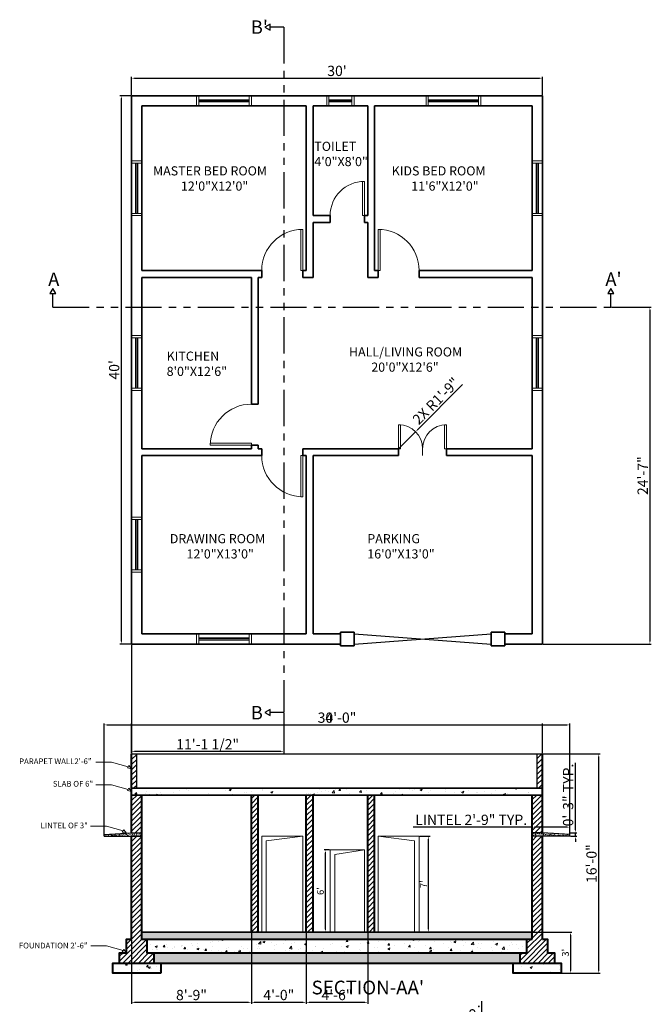
# Model space of a CAD drawing. Units: inches. Extents: x 2639 to 6021, y 292 to 2009.
# Tile 5 of 6: x 3441 to 3995, y 971 to 1833. Entities that reach past the tile are written whole.
import ezdxf

# ---------------------------------------------------------------- set-up
doc = ezdxf.new("R2010")
doc.units = ezdxf.units.IN
doc.linetypes.add('PHANTOM', pattern=[63.5, 31.75, -6.35, 6.35, -6.35, 6.35, -6.35])
for name, color, linetype, lineweight in [('A-ANNO-CUTS', 7, 'PHANTOM', 25), ('A-ANNO-DIMS', 2, 'Continuous', 18), ('A-ANNO-SYMB', 7, 'Continuous', 25), ('A-ANNO-TEXT', 7, 'Continuous', 18), ('A-AREA-IDEN', 7, 'Continuous', 18), ('A-COLS', 7, 'Continuous', 35), ('A-DOOR', 3, 'Continuous', 20), ('A-DOOR-GATE', 3, 'Continuous', 25), ('A-GLAZ', 4, 'Continuous', 18), ('A-ROOF', 7, 'Continuous', 30), ('A-SECT', 7, 'Continuous', 40), ('A-SECT-PATT', 8, 'Continuous', 13), ('A-WALL', 7, 'Continuous', 35), ('S-BEAM', 7, 'Continuous', 30), ('S-FNDN', 7, 'Continuous', 40), ('S-SLAB', 7, 'Continuous', 35)]:
    doc.layers.add(name, color=color, linetype=linetype, lineweight=lineweight)
doc.styles.get("Standard").update_dxf_attribs({"font": 'arial.ttf'})
doc.dimstyles.new('ISO-25', dxfattribs={"dimtxt": 9, "dimasz": 2.5, "dimexe": 1.25, "dimexo": 0.625, "dimtad": 1, "dimdec": 1, "dimlunit": 3, "dimtxsty": 'Standard', "dimcen": 2.5, "dimadec": 0, "dimazin": 0, "dimtfac": 1, "dimtdec": 1, "dimtmove": 0, "dimatfit": 3, "dimfxl": 1, "dimarcsym": 0})
pattern_1 = [(50, (-223.561, 0), (18.218467, -1.59391), [1.905, -20.955]), (355, (-223.561, 0), (-3.52434, 19.105685), [1.524, -16.76406]), (100.45144, (-222.043, -0.133), (14.694125, 17.511775), [1.619, -17.809024]), (46.1842, (-223.56, 5.08), (27.1079, -4.20423), [2.8575, -31.4325]), (96.63556, (-221.302, 4.73), (23.74041, 24.74261), [2.4285, -26.71356]), (351.18415, (-223.56, 5.08), (23.74041, 24.74261), [2.286, -25.14597]), (21, (-221.021, 3.81), (15.16144, -10.22652), [1.905, -20.955]), (326, (-221.021, 3.81), (6.1802, 18.4188), [1.524, -16.764]), (71.45144, (-219.758, 2.958), (21.34164, 8.19228), [1.619, -17.80899]), (37.5, (-223.561, 0), (0.30886, 8.455504), [0, -16.5608, 0, -17.018, 0, -16.8275]), (7.5, (-223.561, 0), (6.681966, 10.018057), [0, -9.7028, 0, -16.1798, 0, -6.4135]), (327.5, (-229.225, 0), (13.55906, -0.572874), [0, -6.35, 0, -19.812, 0, -26.289]), (317.5, (-231.765, 0), (14.812918, 2.54265), [0, -8.255, 0, -13.1572, 0, -18.669])]
pattern_2 = [(50, (-223.561, 0), (1.8218467, -0.15939086), [0.1905, -2.0955]), (355, (-223.561, 0), (-0.3524342, 1.91056845), [0.1524, -1.67640584]), (100.451445, (-223.4092, -0.0133), (1.4694125, 1.7511775), [0.1619001, -1.78090245]), (46.1842, (-223.561, 0.508), (2.7107904, -0.4204233), [0.28575, -3.14325]), (96.63556, (-223.3352, 0.473), (2.3740413, 2.4742612), [0.2428502, -2.671356]), (351.18415, (-223.561, 0.508), (2.3740413, 2.4742612), [0.2285997, -2.5145973]), (21, (-223.307, 0.381), (1.5161439, -1.022652), [0.1905, -2.0955]), (326, (-223.307, 0.381), (0.6180203, 1.8418797), [0.1524, -1.6764]), (71.451445, (-223.1807, 0.2958), (2.1341642, 0.8192277), [0.1619001, -1.7808994]), (37.5, (-223.56106, 0), (0.03088603, 0.84555039), [0, -1.65608, 0, -1.7018, 0, -1.68275]), (7.5, (-223.5611, 0), (0.66819663, 1.00180575), [0, -0.97028, 0, -1.61798, 0, -0.64135]), (327.5, (-224.1275, 0), (1.35590595, -0.05728744), [0, -0.635, 0, -1.9812, 0, -2.6289]), (317.5, (-224.3815, 0), (1.4812918, 0.2542649), [0, -0.8255, 0, -1.31572, 0, -1.8669])]

# ---------------------------------------------------------------- blocks, each defined once
blk = doc.blocks.new('*U2')
for p, q in [((0, 0), (0, -6)), ((30, 0), (30, -6))]:
    blk.add_line(p, q)
blk.add_lwpolyline([(0, 0), (0, 30), (1.75, 30), (1.75, 0)], close=True)
blk.add_arc((0, 0), 30, 0, 90)
blk = doc.blocks.new('*U3')
for p, q in [((0, 0), (0, -6)), ((36, 0), (36, -6))]:
    blk.add_line(p, q)
blk.add_lwpolyline([(0, 0), (0, 36), (1.75, 36), (1.75, 0)], close=True)
blk.add_arc((0, 0), 36, 0, 90)
blk = doc.blocks.new('1')
for p, q in [((0, 6), (0, 0)), ((21, 6), (21, 0)), ((21, 6), (21, 0)), ((42, 6), (42, 0))]:
    blk.add_line(p, q)
for points in [[(0, 6), (0, 27), (1.75, 27), (1.75, 6)], [(42, 6), (42, 27), (40.25, 27), (40.25, 6)]]:
    blk.add_lwpolyline(points, close=True)
for centre, start, end in [((0, 6), 0, 90), ((42, 6), 90, 180)]:
    blk.add_arc(centre, 21, start, end)
blk = doc.blocks.new('*D7')
at = {"layer": 'A-ANNO-DIMS', "color": 0, "lineweight": -2, "transparency": 16777216}
for p, q in [((3538.91, 1766.85), (3529.4, 1766.85)), ((3530.65, 1289.35), (3530.65, 1764.35)), ((3538.91, 1286.85), (3529.4, 1286.85))]:
    blk.add_line(p, q, dxfattribs=at)
at = {"layer": 'A-ANNO-DIMS', "color": 0, "transparency": 16777216}
for points in [[(3530.24, 1764.35), (3531.07, 1764.35), (3530.65, 1766.85)], [(3530.24, 1289.35), (3531.07, 1289.35), (3530.65, 1286.85)]]:
    blk.add_solid(points, dxfattribs=at)
at = {"layer": 'Defpoints', "color": 0, "transparency": 16777216}
for p in [(3530.65, 1766.85), (3539.54, 1766.85), (3539.54, 1286.85)]:
    blk.add_point(p, dxfattribs=at)
at = {"layer": 'A-ANNO-DIMS', "color": 0, "transparency": 16777216, "insert": (3525.43, 1526.85), "char_height": 9, "attachment_point": 5, "rotation": 90}
blk.add_mtext("40'", dxfattribs=at)
blk = doc.blocks.new('*D8')
at = {"layer": 'A-ANNO-DIMS', "color": 0, "lineweight": -2, "transparency": 16777216}
for p, q in [((3539.54, 1767.48), (3539.54, 1783.42)), ((3542.04, 1782.17), (3897.04, 1782.17)), ((3899.54, 1767.48), (3899.54, 1783.42))]:
    blk.add_line(p, q, dxfattribs=at)
at = {"layer": 'A-ANNO-DIMS', "color": 0, "transparency": 16777216}
for points in [[(3542.04, 1782.59), (3542.04, 1781.76), (3539.54, 1782.17)], [(3897.04, 1782.59), (3897.04, 1781.76), (3899.54, 1782.17)]]:
    blk.add_solid(points, dxfattribs=at)
at = {"layer": 'Defpoints', "color": 0, "transparency": 16777216}
for p in [(3899.54, 1782.17), (3539.54, 1766.85), (3899.54, 1766.85)]:
    blk.add_point(p, dxfattribs=at)
at = {"layer": 'A-ANNO-DIMS', "color": 0, "transparency": 16777216, "insert": (3719.54, 1787.4), "char_height": 9, "attachment_point": 5}
blk.add_mtext("30'", dxfattribs=at)
blk = doc.blocks.new('*D15')
at = {"layer": 'A-ANNO-DIMS', "color": 0, "lineweight": -2, "transparency": 16777216}
for p, q in [((3712.91, 1106.63), (3708.23, 1106.63)), ((3709.48, 1037.13), (3709.48, 1104.13)), ((3712.91, 1034.63), (3708.23, 1034.63))]:
    blk.add_line(p, q, dxfattribs=at)
at = {"layer": 'A-ANNO-DIMS', "color": 0, "transparency": 16777216}
for points in [[(3709.06, 1104.13), (3709.89, 1104.13), (3709.48, 1106.63)], [(3709.06, 1037.13), (3709.89, 1037.13), (3709.48, 1034.63)]]:
    blk.add_solid(points, dxfattribs=at)
at = {"layer": 'Defpoints', "color": 0, "transparency": 16777216}
for p in [(3709.48, 1106.63), (3713.54, 1106.63), (3713.54, 1034.63)]:
    blk.add_point(p, dxfattribs=at)
at = {"layer": 'A-ANNO-DIMS', "color": 0, "transparency": 16777216, "insert": (3705.79, 1070.63), "char_height": 6, "attachment_point": 5, "rotation": 90}
blk.add_mtext("6'", dxfattribs=at)
blk = doc.blocks.new('*D16')
at = {"layer": 'A-ANNO-DIMS', "color": 0, "lineweight": -2, "transparency": 16777216}
for p, q in [((3792.16, 1118.63), (3801.09, 1118.63)), ((3799.84, 1037.13), (3799.84, 1116.13)), ((3792.16, 1034.63), (3801.09, 1034.63))]:
    blk.add_line(p, q, dxfattribs=at)
at = {"layer": 'A-ANNO-DIMS', "color": 0, "transparency": 16777216}
for points in [[(3799.43, 1116.13), (3800.26, 1116.13), (3799.84, 1118.63)], [(3799.43, 1037.13), (3800.26, 1037.13), (3799.84, 1034.63)]]:
    blk.add_solid(points, dxfattribs=at)
at = {"layer": 'Defpoints', "color": 0, "transparency": 16777216}
for p in [(3791.54, 1118.63), (3799.84, 1118.63), (3791.54, 1034.63)]:
    blk.add_point(p, dxfattribs=at)
at = {"layer": 'A-ANNO-DIMS', "color": 0, "transparency": 16777216, "insert": (3796.22, 1076.63), "char_height": 6, "attachment_point": 5, "rotation": 90}
blk.add_mtext("7'", dxfattribs=at)
blk = doc.blocks.new('*D17')
at = {"layer": 'A-ANNO-DIMS', "color": 0, "lineweight": -2, "transparency": 16777216}
for p, q in [((3891.16, 1034.63), (3925.39, 1034.63)), ((3924.14, 1032.13), (3924.14, 1001.13)), ((3891.16, 998.63), (3925.39, 998.63))]:
    blk.add_line(p, q, dxfattribs=at)
at = {"layer": 'A-ANNO-DIMS', "color": 0, "transparency": 16777216}
for points in [[(3923.72, 1032.13), (3924.56, 1032.13), (3924.14, 1034.63)], [(3923.72, 1001.13), (3924.56, 1001.13), (3924.14, 998.63)]]:
    blk.add_solid(points, dxfattribs=at)
at = {"layer": 'Defpoints', "color": 0, "transparency": 16777216}
for p in [(3890.54, 1034.63), (3890.54, 998.63), (3924.14, 998.63)]:
    blk.add_point(p, dxfattribs=at)
at = {"layer": 'A-ANNO-DIMS', "color": 0, "transparency": 16777216, "insert": (3920.45, 1016.63), "char_height": 6, "attachment_point": 5, "rotation": 90}
blk.add_mtext("3'", dxfattribs=at)
blk = doc.blocks.new('WINDOW-PLAN-48IN')
for p, q in [((0, 9), (0, 0)), ((44, 9), (44, 0)), ((0, 5.5), (44, 5.5)), ((0, 4.5), (44, 4.5)), ((0, 3.5), (44, 3.5))]:
    blk.add_line(p, q)
blk = doc.blocks.new('WINDOW-PLAN-24IN')
for p, q in [((0, 0), (0, 9)), ((20, 0), (20, 9)), ((0, 5.5), (20, 5.5)), ((0, 4.5), (20, 4.5)), ((0, 3.5), (20, 3.5))]:
    blk.add_line(p, q)
blk = doc.blocks.new('GATE-PIER-12IN')
for p, q in [((0, 12), (12, 12)), ((0, 12), (0, 0)), ((12, 12), (12, 0))]:
    blk.add_line(p, q)
blk.add_lwpolyline([(0, 0), (12, 0)])
blk = doc.blocks.new('GATE-PLAN-10FT')
for p, q in [((0, 9), (120, 0)), ((0, 0), (120, 9))]:
    blk.add_line(p, q)
blk = doc.blocks.new('DOOR-SECTION-36X84')
for p, q in [((0, 0), (0, 84)), ((0, 84), (36, 84)), ((4, 80), (36, 84)), ((4, 0), (4, 80)), ((36, 0), (36, 84))]:
    blk.add_line(p, q)
blk = doc.blocks.new('SECTION-VIEW-ARROW')
blk.add_line((2.6, 0), (2.6, 12))
blk.add_lwpolyline([(2.6, 16.5), (0, 12), (5.2, 12)], close=True)
blk = doc.blocks.new('NOTE-LEADER-SHORT')
blk.add_lwpolyline([(0, 5.93), (13.88, 5.93), (28.37, 1.9)])
blk.add_lwpolyline([(29.01, 2.92), (27.73, 0.89), (31.32, 0)], close=True)
blk = doc.blocks.new('LINTEL-SECTION-33IN')
for p, q in [((0, 1.5), (24, 3)), ((0, 0), (0, 1.5)), ((24, 3), (33, 3)), ((0, 0), (33, 0))]:
    blk.add_line(p, q)
blk = doc.blocks.new('*D44')
at = {"layer": 'A-ANNO-DIMS', "color": 0, "lineweight": -2, "transparency": 16777216}
for p, q in [((3890.54, 1126.58), (3786.21, 1126.58)), ((3890.54, 1122.25), (3890.54, 1127.83)), ((3921.04, 1126.58), (3893.04, 1126.58)), ((3923.54, 1122.25), (3923.54, 1127.83))]:
    blk.add_line(p, q, dxfattribs=at)
at = {"layer": 'A-ANNO-DIMS', "color": 0, "transparency": 16777216}
for points in [[(3893.04, 1127), (3893.04, 1126.16), (3890.54, 1126.58)], [(3921.04, 1127), (3921.04, 1126.16), (3923.54, 1126.58)]]:
    blk.add_solid(points, dxfattribs=at)
at = {"layer": 'Defpoints', "color": 0, "transparency": 16777216}
for p in [(3890.54, 1126.58), (3890.54, 1121.63), (3923.54, 1121.63)]:
    blk.add_point(p, dxfattribs=at)
at = {"layer": 'A-ANNO-DIMS', "color": 0, "transparency": 16777216, "insert": (3837.12, 1131.8), "char_height": 9, "attachment_point": 5}
blk.add_mtext('LINTEL 2\'-9" TYP.', dxfattribs=at)
blk = doc.blocks.new('*D45')
at = {"layer": 'A-ANNO-DIMS', "color": 0, "lineweight": -2, "transparency": 16777216}
for p, q in [((3928.49, 1124.13), (3928.49, 1182.74)), ((3924.16, 1121.63), (3929.74, 1121.63)), ((3928.49, 1118.63), (3928.49, 1121.63)), ((3924.16, 1118.63), (3929.74, 1118.63)), ((3928.49, 1116.13), (3928.49, 1113.63))]:
    blk.add_line(p, q, dxfattribs=at)
at = {"layer": 'A-ANNO-DIMS', "color": 0, "transparency": 16777216}
for points in [[(3928.07, 1124.13), (3928.9, 1124.13), (3928.49, 1121.63)], [(3928.07, 1116.13), (3928.9, 1116.13), (3928.49, 1118.63)]]:
    blk.add_solid(points, dxfattribs=at)
at = {"layer": 'Defpoints', "color": 0, "transparency": 16777216}
for p in [(3923.54, 1121.63), (3928.49, 1121.63), (3923.54, 1118.63)]:
    blk.add_point(p, dxfattribs=at)
at = {"layer": 'A-ANNO-DIMS', "color": 0, "transparency": 16777216, "insert": (3923.26, 1154.68), "char_height": 9, "attachment_point": 5, "rotation": 90}
blk.add_mtext('0\'-3" TYP.', dxfattribs=at)
blk = doc.blocks.new('*D48')
at = {"layer": 'A-ANNO-DIMS', "color": 0, "lineweight": -2, "transparency": 16777216}
for p, q in [((3846.44, 856.63), (3846.44, 974.27)), ((3853.91, 856.63), (3845.19, 856.63)), ((3846.44, 805.13), (3846.44, 854.13)), ((3853.91, 802.63), (3845.19, 802.63))]:
    blk.add_line(p, q, dxfattribs=at)
at = {"layer": 'A-ANNO-DIMS', "color": 0, "transparency": 16777216}
for points in [[(3846.02, 854.13), (3846.85, 854.13), (3846.44, 856.63)], [(3846.02, 805.13), (3846.85, 805.13), (3846.44, 802.63)]]:
    blk.add_solid(points, dxfattribs=at)
at = {"layer": 'Defpoints', "color": 0, "transparency": 16777216}
for p in [(3846.44, 856.63), (3854.54, 856.63), (3854.54, 802.63)]:
    blk.add_point(p, dxfattribs=at)
at = {"layer": 'A-ANNO-DIMS', "color": 0, "transparency": 16777216, "insert": (3841.15, 916.7), "char_height": 9, "attachment_point": 5, "rotation": 90}
blk.add_mtext('WINDOW 4\'-6" TYP.', dxfattribs=at)
blk = doc.blocks.new('*D70')
at = {"layer": 'A-ANNO-DIMS', "color": 0, "lineweight": -2, "transparency": 16777216}
for p, q in [((3539.54, 1286.23), (3539.54, 1191.4)), ((3672.88, 1226.23), (3672.88, 1191.4)), ((3670.38, 1192.65), (3542.04, 1192.65))]:
    blk.add_line(p, q, dxfattribs=at)
at = {"layer": 'A-ANNO-DIMS', "color": 0, "transparency": 16777216}
for points in [[(3542.04, 1193.07), (3542.04, 1192.24), (3539.54, 1192.65)], [(3670.38, 1193.07), (3670.38, 1192.24), (3672.88, 1192.65)]]:
    blk.add_solid(points, dxfattribs=at)
at = {"layer": 'Defpoints', "color": 0, "transparency": 16777216}
for p in [(3539.54, 1286.85), (3672.88, 1226.85), (3539.54, 1192.65)]:
    blk.add_point(p, dxfattribs=at)
at = {"layer": 'A-ANNO-DIMS', "color": 0, "transparency": 16777216, "insert": (3606.21, 1197.93), "char_height": 9, "attachment_point": 5}
blk.add_mtext('11\'-1 1/2"', dxfattribs=at)
blk = doc.blocks.new('*D71')
at = {"layer": 'A-ANNO-DIMS', "color": 0, "lineweight": -2, "transparency": 16777216}
for p, q in [((3960.16, 1581.68), (3994.98, 1581.68)), ((3993.73, 1579.18), (3993.73, 1289.35)), ((3900.16, 1286.85), (3994.98, 1286.85))]:
    blk.add_line(p, q, dxfattribs=at)
at = {"layer": 'A-ANNO-DIMS', "color": 0, "transparency": 16777216}
for points in [[(3993.32, 1579.18), (3994.15, 1579.18), (3993.73, 1581.68)], [(3993.32, 1289.35), (3994.15, 1289.35), (3993.73, 1286.85)]]:
    blk.add_solid(points, dxfattribs=at)
at = {"layer": 'Defpoints', "color": 0, "transparency": 16777216}
for p in [(3959.54, 1581.68), (3899.54, 1286.85), (3993.73, 1286.85)]:
    blk.add_point(p, dxfattribs=at)
at = {"layer": 'A-ANNO-DIMS', "color": 0, "transparency": 16777216, "insert": (3988.59, 1434.26), "char_height": 9, "attachment_point": 5, "rotation": 90}
blk.add_mtext('24\'-7"', dxfattribs=at)
blk = doc.blocks.new('*D98')
at = {"layer": 'A-ANNO-DIMS', "color": 0, "lineweight": -2, "transparency": 16777216}
for p, q in [((3515.54, 1119.25), (3515.54, 1217.28)), ((3518.04, 1216.03), (3921.04, 1216.03)), ((3923.54, 1119.25), (3923.54, 1217.28))]:
    blk.add_line(p, q, dxfattribs=at)
at = {"layer": 'A-ANNO-DIMS', "color": 0, "transparency": 16777216}
for points in [[(3518.04, 1216.45), (3518.04, 1215.61), (3515.54, 1216.03)], [(3921.04, 1216.45), (3921.04, 1215.61), (3923.54, 1216.03)]]:
    blk.add_solid(points, dxfattribs=at)
at = {"layer": 'Defpoints', "color": 0, "transparency": 16777216}
for p in [(3923.54, 1216.03), (3515.54, 1118.63), (3923.54, 1118.63)]:
    blk.add_point(p, dxfattribs=at)
at = {"layer": 'A-ANNO-DIMS', "color": 0, "transparency": 16777216, "insert": (3719.54, 1221.25), "char_height": 9, "attachment_point": 5}
blk.add_mtext('34\'-0"', dxfattribs=at)
blk = doc.blocks.new('*D99')
at = {"layer": 'A-ANNO-DIMS', "color": 0, "lineweight": -2, "transparency": 16777216}
for p, q in [((3539.54, 1191.25), (3539.54, 1217.28)), ((3542.04, 1216.03), (3897.04, 1216.03)), ((3899.54, 1191.25), (3899.54, 1217.28))]:
    blk.add_line(p, q, dxfattribs=at)
at = {"layer": 'A-ANNO-DIMS', "color": 0, "transparency": 16777216}
for points in [[(3542.04, 1216.45), (3542.04, 1215.61), (3539.54, 1216.03)], [(3897.04, 1216.45), (3897.04, 1215.61), (3899.54, 1216.03)]]:
    blk.add_solid(points, dxfattribs=at)
at = {"layer": 'Defpoints', "color": 0, "transparency": 16777216}
for p in [(3899.54, 1216.03), (3539.54, 1190.63), (3899.54, 1190.63)]:
    blk.add_point(p, dxfattribs=at)
at = {"layer": 'A-ANNO-DIMS', "color": 0, "transparency": 16777216, "insert": (3719.54, 1221.25), "char_height": 9, "attachment_point": 5}
blk.add_mtext('30\'-0"', dxfattribs=at)
blk = doc.blocks.new('*D100')
at = {"layer": 'A-ANNO-DIMS', "color": 0, "lineweight": -2, "transparency": 16777216}
for p, q in [((3900.16, 1190.63), (3950.19, 1190.63)), ((3948.94, 1001.13), (3948.94, 1188.13)), ((3916.66, 998.63), (3950.19, 998.63))]:
    blk.add_line(p, q, dxfattribs=at)
at = {"layer": 'A-ANNO-DIMS', "color": 0, "transparency": 16777216}
for points in [[(3948.52, 1188.13), (3949.35, 1188.13), (3948.94, 1190.63)], [(3948.52, 1001.13), (3949.35, 1001.13), (3948.94, 998.63)]]:
    blk.add_solid(points, dxfattribs=at)
at = {"layer": 'Defpoints', "color": 0, "transparency": 16777216}
for p in [(3899.54, 1190.63), (3948.94, 1190.63), (3916.04, 998.63)]:
    blk.add_point(p, dxfattribs=at)
at = {"layer": 'A-ANNO-DIMS', "color": 0, "transparency": 16777216, "insert": (3943.72, 1094.63), "char_height": 9, "attachment_point": 5, "rotation": 90}
blk.add_mtext('16\'-0"', dxfattribs=at)
blk = doc.blocks.new('*D101')
at = {"layer": 'A-ANNO-DIMS', "color": 0, "lineweight": -2, "transparency": 16777216}
for p, q in [((3539.54, 1028), (3539.54, 971.98)), ((3644.54, 1034), (3644.54, 971.98)), ((3542.04, 973.23), (3642.04, 973.23))]:
    blk.add_line(p, q, dxfattribs=at)
at = {"layer": 'A-ANNO-DIMS', "color": 0, "transparency": 16777216}
for points in [[(3542.04, 973.65), (3542.04, 972.81), (3539.54, 973.23)], [(3642.04, 973.65), (3642.04, 972.81), (3644.54, 973.23)]]:
    blk.add_solid(points, dxfattribs=at)
at = {"layer": 'Defpoints', "color": 0, "transparency": 16777216}
for p in [(3644.54, 1034.63), (3539.54, 1028.63), (3644.54, 973.23)]:
    blk.add_point(p, dxfattribs=at)
at = {"layer": 'A-ANNO-DIMS', "color": 0, "transparency": 16777216, "insert": (3592.04, 978.45), "char_height": 9, "attachment_point": 5}
blk.add_mtext('8\'-9"', dxfattribs=at)
blk = doc.blocks.new('*D102')
at = {"layer": 'A-ANNO-DIMS', "color": 0, "lineweight": -2, "transparency": 16777216}
for p, q in [((3644.54, 1034), (3644.54, 971.98)), ((3692.54, 1034), (3692.54, 971.98)), ((3647.04, 973.23), (3690.04, 973.23))]:
    blk.add_line(p, q, dxfattribs=at)
at = {"layer": 'A-ANNO-DIMS', "color": 0, "transparency": 16777216}
for points in [[(3647.04, 973.65), (3647.04, 972.81), (3644.54, 973.23)], [(3690.04, 973.65), (3690.04, 972.81), (3692.54, 973.23)]]:
    blk.add_solid(points, dxfattribs=at)
at = {"layer": 'Defpoints', "color": 0, "transparency": 16777216}
for p in [(3644.54, 1034.63), (3692.54, 1034.63), (3692.54, 973.23)]:
    blk.add_point(p, dxfattribs=at)
at = {"layer": 'A-ANNO-DIMS', "color": 0, "transparency": 16777216, "insert": (3668.54, 978.45), "char_height": 9, "attachment_point": 5}
blk.add_mtext('4\'-0"', dxfattribs=at)
blk = doc.blocks.new('*D103')
at = {"layer": 'A-ANNO-DIMS', "color": 0, "lineweight": -2, "transparency": 16777216}
for p, q in [((3692.54, 1034), (3692.54, 971.98)), ((3746.54, 1034), (3746.54, 971.98)), ((3695.04, 973.23), (3744.04, 973.23))]:
    blk.add_line(p, q, dxfattribs=at)
at = {"layer": 'A-ANNO-DIMS', "color": 0, "transparency": 16777216}
for points in [[(3695.04, 973.65), (3695.04, 972.81), (3692.54, 973.23)], [(3744.04, 973.65), (3744.04, 972.81), (3746.54, 973.23)]]:
    blk.add_solid(points, dxfattribs=at)
at = {"layer": 'Defpoints', "color": 0, "transparency": 16777216}
for p in [(3692.54, 1034.63), (3746.54, 1034.63), (3746.54, 973.23)]:
    blk.add_point(p, dxfattribs=at)
at = {"layer": 'A-ANNO-DIMS', "color": 0, "transparency": 16777216, "insert": (3719.54, 978.45), "char_height": 9, "attachment_point": 5}
blk.add_mtext('4\'-6"', dxfattribs=at)
blk = doc.blocks.new('*D113')
at = {"layer": 'A-ANNO-DIMS', "color": 0, "lineweight": -2, "transparency": 16777216}
for p, q in [((3829.59, 1513.91), (3790.15, 1474.47)), ((3773.54, 1457.85), (3788.38, 1472.7))]:
    blk.add_line(p, q, dxfattribs=at)
at = {"layer": 'A-ANNO-DIMS', "color": 0, "transparency": 16777216}
blk.add_solid([(3789.86, 1474.76), (3790.45, 1474.17), (3788.38, 1472.7)], dxfattribs=at)
at = {"layer": 'Defpoints', "color": 0, "transparency": 16777216}
for p in [(3788.38, 1472.7), (3773.54, 1457.85)]:
    blk.add_point(p, dxfattribs=at)
at = {"layer": 'A-ANNO-DIMS', "color": 0, "transparency": 16777216, "insert": (3807.07, 1498.76), "char_height": 9, "attachment_point": 5, "rotation": 45.00041}
blk.add_mtext('2X R1\'-9"', dxfattribs=at)

msp = doc.modelspace()

# ---------------------------------------------------------------- hatches: boundary and pattern name
at = {"layer": 'A-SECT-PATT'}
h = msp.add_hatch(dxfattribs=at)
h.set_pattern_fill('ANSI31', color=256)
h.set_pattern_definition([(45, (-223.561, 0), (-2.245064, 2.245064), [])])
h.paths.add_polyline_path([(3548.54, 1154.63), (3539.54, 1154.63), (3539.54, 1121.63), (3548.54, 1121.63)])
h.paths.add_polyline_path([(3548.54, 1118.63), (3539.54, 1118.63), (3539.54, 1028.63), (3535.04, 1028.63), (3535.04, 1016.63), (3529.04, 1016.63), (3529.04, 1007.63), (3559.04, 1007.63), (3559.04, 1016.63), (3553.04, 1016.63), (3553.04, 1028.63), (3548.54, 1028.63)])
h.paths.add_polyline_path([(3544.04, 1190.63), (3539.54, 1190.63), (3539.54, 1160.63), (3544.04, 1160.63)])
h.paths.add_polyline_path([(3650.54, 1154.63), (3644.54, 1154.63), (3644.54, 1034.63), (3650.54, 1034.63)])
h.paths.add_polyline_path([(3698.54, 1154.63), (3692.54, 1154.63), (3692.54, 1034.63), (3698.54, 1034.63)])
h.paths.add_polyline_path([(3752.54, 1154.63), (3746.54, 1154.63), (3746.54, 1034.63), (3752.54, 1034.63)])
h.paths.add_polyline_path([(3899.54, 1190.63), (3895.04, 1190.63), (3895.04, 1160.63), (3899.54, 1160.63)])
h.paths.add_polyline_path([(3899.54, 1154.63), (3890.54, 1154.63), (3890.54, 1121.63), (3899.54, 1121.63)])
h.paths.add_polyline_path([(3899.54, 1118.63), (3890.54, 1118.63), (3890.54, 1028.63), (3886.04, 1028.63), (3886.04, 1016.63), (3880.04, 1016.63), (3880.04, 1007.63), (3910.04, 1007.63), (3910.04, 1016.63), (3904.04, 1016.63), (3904.04, 1028.63), (3899.54, 1028.63)])
h = msp.add_hatch(dxfattribs=at)
h.set_pattern_fill('AR-CONC', color=256, scale=0.1)
h.set_pattern_definition(pattern_1)
h.paths.add_polyline_path([(3899.54, 1160.63), (3539.54, 1160.63), (3539.54, 1154.63), (3899.54, 1154.63)])
h = msp.add_hatch(dxfattribs=at)
h.set_pattern_fill('AR-CONC', color=256, scale=0.01)
h.set_pattern_definition(pattern_2)
h.paths.add_polyline_path([(3548.54, 1121.63), (3539.54, 1121.63), (3515.54, 1120.13), (3515.54, 1118.63), (3548.54, 1118.63)])
h = msp.add_hatch(dxfattribs=at)
h.set_pattern_fill('AR-CONC', color=256, scale=0.01)
h.set_pattern_definition(pattern_2)
h.paths.add_polyline_path([(3899.54, 1121.63), (3890.54, 1121.63), (3890.54, 1118.63), (3923.54, 1118.63), (3923.54, 1120.13)])
h = msp.add_hatch(dxfattribs=at)
h.set_pattern_fill('AR-SAND', color=256, scale=0.1)
h.set_pattern_definition([(37.5, (-223.561, 0), (-0.160003, 4.8941324), [0, -3.8608, 0, -4.318, 0, -4.1275]), (7.5, (-223.561, 0), (4.495233, 7.168251), [0, -2.0828, 0, -3.4798, 0, -1.3335]), (327.5, (-226.6853, 0), (7.9099237, 0.014372), [0, -1.27, 0, -4.572, 0, -5.969]), (317.5, (-226.685, 0), (7.635565, 2.229293), [0, -0.635, 0, -2.9972, 0, -3.429])])
h.paths.add_polyline_path([(3890.54, 1034.63), (3548.54, 1034.63), (3548.54, 1028.63), (3553.04, 1028.63), (3886.04, 1028.63), (3890.54, 1028.63)])
h = msp.add_hatch(dxfattribs=at)
h.set_pattern_fill('AR-CONC', color=256, scale=0.1)
h.set_pattern_definition(pattern_1)
h.paths.add_polyline_path([(3880.04, 1016.63), (3886.04, 1016.63), (3886.04, 1028.63), (3553.04, 1028.63), (3553.04, 1016.63), (3559.04, 1016.63)])
h = msp.add_hatch(dxfattribs=at)
h.set_pattern_fill('GRAVEL', color=256, scale=0.5)
h.set_pattern_definition([(228.012788, (-214.4171, 12.7), (-101.6, -114.3), [1.708607, -169.15242]), (184.969741, (-215.56006, 11.43), (152.39999994, 12.70000072), [2.932024, -290.270244]), (132.510447, (-218.48106, 11.176), (127.00000005, -139.69999995), [2.067408, -204.673614]), (267.273689, (-223.43406, 8.001), (12.70000003, 254), [2.670023, -264.332187]), (292.833654, (-223.56106, 5.334), (-63.500000005, 152.4), [2.61817, -259.19904]), (357.273689, (-222.54506, 2.921), (-254, 12.70000003), [2.670023, -264.332187]), (37.69424, (-219.87806, 2.794), (-165.099999993, -127.00000001), [3.53097, -349.565577]), (72.255328, (-217.08406, 4.953), (88.900000024, 279.39999999), [3.333598, -330.026283]), (121.429566, (-216.06806, 8.128), (-101.600000014, 165.09999999), [2.679065, -265.22773]), (175.236358, (-217.4651, 10.414), (139.7, -12.70000002), [3.058566, -149.869685]), (222.397438, (-220.51306, 10.668), (-152.399999995, -139.700000005), [3.95539, -391.583863]), (138.814075, (-210.861, 7.874), (-88.9, 76.2), [1.350023, -133.65283]), (171.469234, (-211.87706, 8.763), (165.1, -25.39999997), [2.56841, -254.273195]), (225, (-214.417, 9.144), (-2e-15, -12.7), [1.796047, -16.164466]), (203.19859, (-215.306, 10.668), (63.5, 25.4), [0.967207, -95.75311]), (291.80141, (-216.195, 10.287), (-12.7, 38.1), [1.367828, -67.023765]), (30.963757, (-215.687, 9.017), (38.1, 25.4), [2.2216, -71.83149]), (161.56505, (-213.782, 10.16), (25.4, -12.7), [1.606436, -38.55449]), (16.38954, (-223.56106, 10.287), (127, 38.1), [2.25044, -222.794133]), (70.346176, (-221.40206, 10.922), (-50.8, -139.7), [1.887995, -186.91108]), (293.19859, (-213.782, 12.7), (-25.4, 63.5), [1.9344, -94.785918]), (343.61046, (-213.02006, 10.922), (-127, 38.09999999), [2.25044, -222.794133]), (339.443955, (-223.561, 2.413), (-63.5, 25.4), [2.170176, -106.33867]), (294.77514, (-221.5291, 1.651), (-63.50000008, 139.69999997), [1.81836, -180.017967]), (66.80141, (-213.655, 0), (25.4, 63.5), [1.9344, -94.785918]), (17.354025, (-212.89306, 1.778), (-165.1, -50.80000001), [2.128914, -210.76188]), (69.443955, (-219.878, 0), (-25.4, -63.5), [1.085088, -107.42376]), (101.30993, (-214.417, 0), (-12.7, 50.8), [0.647573, -64.109975]), (165.96376, (-214.544, 0.635), (38.1, -12.7), [2.61817, -49.745273]), (186.009006, (-217.08406, 1.27), (127, 12.70000001), [2.426335, -240.206824]), (303.69007, (-215.687, 7.874), (-12.7, 25.4), [1.83162, -43.95888]), (353.157227, (-214.67106, 6.35), (215.9, -25.39999999), [3.197784, -316.580045]), (60.945396, (-211.496, 5.969), (-50.8, -88.9), [1.30754, -129.44696]), (90, (-210.861, 7.112), (-12.7, 12.7), [0.762, -11.938]), (120.256437, (-217.3381, 1.651), (50.8, -88.9), [1.764335, -174.669704]), (48.012787, (-218.2271, 3.175), (101.6, 114.3), [3.417214, -167.44381]), (0, (-215.941, 5.715), (12.7, 12.7), [3.302, -9.398]), (325.304846, (-212.63906, 5.715), (127.00000005, -88.89999993), [2.008048, -198.796584]), (254.054604, (-210.988, 4.572), (-12.7, -50.8), [1.849145, -90.60825]), (207.645975, (-211.49606, 2.794), (-241.30000001, -126.99999998), [3.010725, -298.062322]), (175.426079, (-214.16306, 1.397), (-165.1, 12.7), [3.185147, -315.329232])])
h.paths.add_polyline_path([(3874.04, 1007.63), (3880.04, 1007.63), (3880.04, 1016.63), (3559.04, 1016.63), (3559.04, 1007.63), (3565.04, 1007.63)])
h = msp.add_hatch(dxfattribs=at)
h.set_pattern_fill('AR-CONC', color=256, scale=0.1)
h.set_pattern_definition(pattern_1)
h.paths.add_polyline_path([(3565.04, 998.63), (3565.04, 1007.63), (3559.04, 1007.63), (3529.04, 1007.63), (3523.04, 1007.63), (3523.04, 998.63)])
h.paths.add_polyline_path([(3916.04, 998.63), (3916.04, 1007.63), (3910.04, 1007.63), (3880.04, 1007.63), (3874.04, 1007.63), (3874.04, 998.63)])

# ---------------------------------------------------------------- linework, layer by layer
at = {"layer": 'A-ANNO-CUTS'}
for p, q in [((3672.88, 1826.85), (3672.88, 1226.85)), ((3470.65, 1581.68), (3959.54, 1581.68))]:
    msp.add_line(p, q, dxfattribs=at)
at = {"layer": 'A-DOOR'}
for p, q in [((3713.54, 1034.63), (3713.54, 1106.63)), ((3713.54, 1106.63), (3743.54, 1106.63)), ((3717.54, 1102.63), (3743.54, 1106.63)), ((3743.54, 1034.63), (3743.54, 1106.63)), ((3717.54, 1034.63), (3717.54, 1102.63))]:
    msp.add_line(p, q, dxfattribs=at)
at = {"layer": 'A-GLAZ'}
for p, q in [((3596.54, 1757.85), (3596.54, 1766.85)), ((3644.54, 1757.85), (3644.54, 1766.85)), ((3710.54, 1757.85), (3710.54, 1766.85)), ((3734.54, 1757.85), (3734.54, 1766.85)), ((3797.54, 1757.85), (3797.54, 1766.85)), ((3845.54, 1757.85), (3845.54, 1766.85)), ((3548.54, 1709.85), (3539.54, 1709.85)), ((3890.54, 1709.85), (3899.54, 1709.85)), ((3548.54, 1661.85), (3539.54, 1661.85)), ((3890.54, 1661.85), (3899.54, 1661.85)), ((3548.54, 1556.85), (3539.54, 1556.85)), ((3890.54, 1556.85), (3899.54, 1556.85)), ((3548.54, 1508.85), (3539.54, 1508.85)), ((3890.54, 1508.85), (3899.54, 1508.85)), ((3548.54, 1397.85), (3539.54, 1397.85)), ((3548.54, 1349.85), (3539.54, 1349.85)), ((3596.54, 1295.85), (3596.54, 1286.85)), ((3644.54, 1295.85), (3644.54, 1286.85))]:
    msp.add_line(p, q, dxfattribs=at)
at = {"layer": 'A-ROOF'}
for p, q in [((3539.54, 1190.63), (3899.54, 1190.63)), ((3544.04, 1160.63), (3544.04, 1190.63)), ((3895.04, 1160.63), (3895.04, 1190.63))]:
    msp.add_line(p, q, dxfattribs=at)
at = {"layer": 'A-SECT'}
for p, q in [((3539.54, 1121.63), (3539.54, 1190.63)), ((3899.54, 1121.63), (3899.54, 1190.63)), ((3548.54, 1028.63), (3548.54, 1154.63)), ((3644.54, 1034.63), (3644.54, 1154.63)), ((3650.54, 1034.63), (3650.54, 1154.63)), ((3692.54, 1034.63), (3692.54, 1154.63)), ((3698.54, 1034.63), (3698.54, 1154.63)), ((3746.54, 1034.63), (3746.54, 1154.63)), ((3752.54, 1034.63), (3752.54, 1154.63)), ((3890.54, 1028.63), (3890.54, 1154.63)), ((3539.54, 1028.63), (3539.54, 1118.63)), ((3899.54, 1028.63), (3899.54, 1118.63))]:
    msp.add_line(p, q, dxfattribs=at)
at = {"layer": 'A-WALL'}
for p, q in [((3692.54, 1757.85), (3548.54, 1757.85)), ((3548.54, 1757.85), (3548.54, 1613.85)), ((3692.54, 1757.85), (3692.54, 1613.85)), ((3746.54, 1757.85), (3698.54, 1757.85)), ((3698.54, 1757.85), (3698.54, 1661.85)), ((3746.54, 1757.85), (3746.54, 1661.85)), ((3890.54, 1757.85), (3752.54, 1757.85)), ((3752.54, 1757.85), (3752.54, 1613.85)), ((3890.54, 1613.85), (3890.54, 1757.85)), ((3713.54, 1661.85), (3698.54, 1661.85)), ((3713.54, 1655.85), (3698.54, 1655.85)), ((3698.54, 1655.85), (3698.54, 1607.85)), ((3713.54, 1661.85), (3713.54, 1655.85)), ((3746.54, 1661.85), (3743.54, 1661.85)), ((3743.54, 1661.85), (3743.54, 1655.85)), ((3746.54, 1655.85), (3743.54, 1655.85)), ((3746.54, 1655.85), (3746.54, 1607.85)), ((3653.54, 1613.85), (3548.54, 1613.85)), ((3653.54, 1613.85), (3653.54, 1607.85)), ((3692.54, 1613.85), (3689.54, 1613.85)), ((3689.54, 1613.85), (3689.54, 1607.85)), ((3755.54, 1613.85), (3752.54, 1613.85)), ((3755.54, 1613.85), (3755.54, 1607.85)), ((3890.54, 1613.85), (3791.54, 1613.85)), ((3791.54, 1613.85), (3791.54, 1607.85)), ((3644.54, 1607.85), (3548.54, 1607.85)), ((3548.54, 1607.85), (3548.54, 1457.85)), ((3644.54, 1607.85), (3644.54, 1496.85)), ((3653.54, 1607.85), (3650.54, 1607.85)), ((3650.54, 1607.85), (3650.54, 1496.85)), ((3698.54, 1607.85), (3689.54, 1607.85)), ((3755.54, 1607.85), (3746.54, 1607.85)), ((3890.54, 1607.85), (3791.54, 1607.85)), ((3890.54, 1457.85), (3890.54, 1607.85)), ((3650.54, 1496.85), (3644.54, 1496.85)), ((3644.54, 1457.85), (3548.54, 1457.85)), ((3650.54, 1460.85), (3644.54, 1460.85)), ((3644.54, 1460.85), (3644.54, 1457.85)), ((3650.54, 1460.85), (3650.54, 1457.85)), ((3653.54, 1457.85), (3650.54, 1457.85)), ((3653.54, 1457.85), (3653.54, 1451.85)), ((3773.54, 1457.85), (3689.54, 1457.85)), ((3689.54, 1457.85), (3689.54, 1451.85)), ((3773.54, 1451.85), (3773.54, 1457.85)), ((3890.54, 1457.85), (3815.54, 1457.85)), ((3815.54, 1451.85), (3815.54, 1457.85)), ((3653.54, 1451.85), (3548.54, 1451.85)), ((3548.54, 1451.85), (3548.54, 1295.85)), ((3692.54, 1451.85), (3689.54, 1451.85)), ((3692.54, 1451.85), (3692.54, 1295.85)), ((3773.54, 1451.85), (3698.54, 1451.85)), ((3698.54, 1451.85), (3698.54, 1295.85)), ((3890.54, 1451.85), (3815.54, 1451.85)), ((3890.54, 1295.85), (3890.54, 1451.85)), ((3548.54, 1295.85), (3692.54, 1295.85)), ((3698.54, 1295.85), (3722.54, 1295.85)), ((3866.54, 1295.85), (3890.54, 1295.85))]:
    msp.add_line(p, q, dxfattribs=at)
msp.add_lwpolyline([(3866.54, 1286.85), (3899.54, 1286.85), (3899.54, 1766.85), (3539.54, 1766.85), (3539.54, 1286.85), (3722.54, 1286.85)], dxfattribs=at)
at = {"layer": 'S-FNDN'}
for p, q in [((3548.54, 1028.63), (3886.04, 1028.63)), ((3559.04, 1016.63), (3880.04, 1016.63)), ((3529.04, 1007.63), (3559.04, 1007.63)), ((3565.04, 1007.63), (3874.04, 1007.63)), ((3880.04, 1007.63), (3910.04, 1007.63))]:
    msp.add_line(p, q, dxfattribs=at)
for points in [[(3565.04, 998.63), (3523.04, 998.63), (3523.04, 1007.63), (3529.04, 1007.63), (3529.04, 1016.63), (3535.04, 1016.63), (3535.04, 1028.63), (3539.54, 1028.63)], [(3548.54, 1028.63), (3553.04, 1028.63), (3553.04, 1016.63), (3559.04, 1016.63), (3559.04, 1007.63), (3565.04, 1007.63), (3565.04, 998.63)], [(3916.04, 998.63), (3874.04, 998.63), (3874.04, 1007.63), (3880.04, 1007.63), (3880.04, 1016.63), (3886.04, 1016.63), (3886.04, 1028.63), (3890.54, 1028.63)], [(3899.54, 1028.63), (3904.04, 1028.63), (3904.04, 1016.63), (3910.04, 1016.63), (3910.04, 1007.63), (3916.04, 1007.63), (3916.04, 998.63)]]:
    msp.add_lwpolyline(points, dxfattribs=at)
at = {"layer": 'S-SLAB'}
for p, q in [((3539.54, 1160.63), (3899.54, 1160.63)), ((3539.54, 1154.63), (3899.54, 1154.63)), ((3548.54, 1034.63), (3890.54, 1034.63))]:
    msp.add_line(p, q, dxfattribs=at)

# ---------------------------------------------------------------- block references
at = {"layer": 'A-ANNO-SYMB', "rotation": 89.99999999999886}
for p in [(3672.88, 1824.25), (3672.88, 1224.25)]:
    msp.add_blockref('SECTION-VIEW-ARROW', p, dxfattribs=at)
at = {"layer": 'A-ANNO-SYMB'}
for p in [(3468.05, 1581.68), (3956.94, 1581.68)]:
    msp.add_blockref('SECTION-VIEW-ARROW', p, dxfattribs=at)
at = {"layer": 'A-ANNO-TEXT'}
for p in [(3508.21, 1177.51), (3508.21, 1157.64), (3503.68, 1121.35), (3503.71, 1016.63)]:
    msp.add_blockref('NOTE-LEADER-SHORT', p, dxfattribs=at)
at = {"layer": 'A-COLS'}
msp.add_blockref('GATE-PIER-12IN', (3722.54, 1285.35), dxfattribs=at)
at = {"layer": 'A-COLS', "rotation": 180}
msp.add_blockref('GATE-PIER-12IN', (3866.54, 1297.35), dxfattribs=at)
at = {"layer": 'A-DOOR', "xscale": -1}
for name, p in [('*U2', (3743.54, 1661.85)), ('*U3', (3689.54, 1613.85))]:
    msp.add_blockref(name, p, dxfattribs=at)
at = {"layer": 'A-DOOR'}
for name, p in [('*U3', (3755.54, 1613.85)), ('1', (3773.54, 1451.85)), ('DOOR-SECTION-36X84', (3653.54, 1034.63))]:
    msp.add_blockref(name, p, dxfattribs=at)
for p, rotation in [((3644.54, 1460.84), 90), ((3689.54, 1451.85), 180)]:
    msp.add_blockref('*U3', p, dxfattribs=dict(at, rotation=rotation))
at = {"layer": 'A-DOOR', "extrusion": (0, 0, -1), "zscale": -1}
msp.add_blockref('DOOR-SECTION-36X84', (-3791.54, 1034.63), dxfattribs=at)
at = {"layer": 'A-DOOR-GATE'}
msp.add_blockref('GATE-PLAN-10FT', (3734.54, 1286.85), dxfattribs=at)
at = {"layer": 'A-GLAZ'}
for name, p in [('WINDOW-PLAN-48IN', (3598.54, 1757.85)), ('WINDOW-PLAN-24IN', (3712.54, 1757.85)), ('WINDOW-PLAN-48IN', (3799.54, 1757.85)), ('WINDOW-PLAN-48IN', (3598.54, 1286.85))]:
    msp.add_blockref(name, p, dxfattribs=at)
for p, rotation in [((3539.54, 1707.85), 269.9999999999988), ((3890.54, 1707.85), 269.9999999999988), ((3548.54, 1510.85), 89.99999999999876), ((3890.54, 1554.85), 269.9999999999998), ((3548.54, 1351.85), 89.99999999999841)]:
    msp.add_blockref('WINDOW-PLAN-48IN', p, dxfattribs=dict(at, rotation=rotation))
at = {"layer": 'S-BEAM'}
msp.add_blockref('LINTEL-SECTION-33IN', (3515.54, 1118.63), dxfattribs=at)
at = {"layer": 'S-BEAM', "extrusion": (0, 0, -1), "zscale": -1}
msp.add_blockref('LINTEL-SECTION-33IN', (-3923.54, 1118.63), dxfattribs=at)

# ---------------------------------------------------------------- texts
at = {"layer": 'A-ANNO-SYMB'}
for s, height, p in [("B'", 11.732, (3644.06, 1821.04)), ('A', 11.73, (3466.5, 1600.35)), ("A'", 11.732, (3954.73, 1600.35)), ('B', 11.73, (3644.06, 1220.87))]:
    msp.add_text(s, height=height, dxfattribs=at).set_placement(p)
at = {"layer": 'A-ANNO-TEXT', "attachment_point": 1}
for s, width, heights, insert, char_height in [('{\\fTimes New Roman|b0|i0|c0|p18;PARAPET WALL2\'-6"}', 172.2916, [0], (3440.99, 1186.7), 5), ('{\\fTimes New Roman|b0|i0|c0|p18;SLAB OF 6"}', 40.7521, [5.11], (3470.53, 1167.04), 5), ('{\\fTimes New Roman|b0|i0|c0|p18;LINTEL OF 3"}', 49.0691, [0], (3459.87, 1130.53), 5), ('{\\fTimes New Roman|b0|i0|c0|p18;FOUNDATION 2\'-6"}', 65.4654, [0], (3440.8, 1025.39), 5), ("{\\fTimes New Roman|b0|i0|c0|p18;SECTION-AA'}", 172.2916, [0], (3697.3, 992.17), 12)]:
    msp.add_mtext_dynamic_manual_height_columns(s, width=width, gutter_width=12.5, heights=heights, dxfattribs=dict(at, insert=insert, char_height=char_height))
at = {"layer": 'A-AREA-IDEN', "char_height": 8, "attachment_point": 1}
for s, insert in [('{\\fTimes New Roman|b0|i0|c0|p18;TOILET\\P4\'0"X8\'0"}', (3699.69, 1726.52)), ('{\\fTimes New Roman|b0|i0|c0|p18;MASTER BED ROOM\\P          12\'0"X12\'0"}', (3558.34, 1705.05)), ('{\\fTimes New Roman|b0|i0|c0|p18;KIDS BED ROOM\\P       11\'6"X12\'0"}', (3767.52, 1705.05)), ('{\\fTimes New Roman|b0|i0|c0|p18;KITCHEN\\P8\'0"X12\'6"}', (3570.29, 1542.86)), ('{\\fTimes New Roman|b0|i0|c0|p18;HALL/LIVING ROOM\\P        20\'0"X12\'6"}', (3730.06, 1546.56)), ('{\\fTimes New Roman|b0|i0|c0|p18;DRAWING ROOM\\P      12\'0"X13\'0"}', (3573.04, 1383.08)), ('{\\fTimes New Roman|b0|i0|c0|p18;PARKING\\P16\'0"X13\'0"}', (3746.12, 1383.08))]:
    msp.add_mtext_dynamic_manual_height_columns(s, width=172.2916, gutter_width=12.5, heights=[0], dxfattribs=dict(at, insert=insert))

# ---------------------------------------------------------------- dimensions: what is measured, and where the dimension line sits
at = {"layer": 'A-ANNO-DIMS'}
for base, p1, p2, override, picture, middle in [((3899.54, 1782.17), (3539.54, 1766.85), (3899.54, 1766.85), {"dimclrd": 0, "dimclre": 0, "dimclrt": 0}, '*D8', (3719.54, 1787.4)), ((3539.54, 1192.65), (3672.88, 1226.85), (3539.54, 1286.85), {"dimdec": 1, "dimlfac": 1, "dimrnd": 0, "dimzin": 1, "dimdsep": 46, "dimlunit": 4, "dimfrac": 2}, '*D70', (3606.21, 1197.93)), ((3923.54, 1216.03), (3515.54, 1118.63), (3923.54, 1118.63), {"dimdec": 1, "dimlfac": 1, "dimrnd": 0, "dimzin": 1, "dimdsep": 46, "dimlunit": 4, "dimfrac": 2}, '*D98', (3719.54, 1221.25)), ((3899.54, 1216.03), (3539.54, 1190.63), (3899.54, 1190.63), {"dimdec": 1, "dimlfac": 1, "dimrnd": 0, "dimzin": 1, "dimdsep": 46, "dimlunit": 4, "dimfrac": 2}, '*D99', (3719.54, 1221.25)), ((3644.54, 973.23), (3539.54, 1028.63), (3644.54, 1034.63), {"dimdec": 1, "dimlfac": 1, "dimrnd": 0, "dimzin": 1, "dimdsep": 46, "dimlunit": 4, "dimfrac": 2}, '*D101', (3592.04, 978.45)), ((3692.54, 973.23), (3644.54, 1034.63), (3692.54, 1034.63), {"dimdec": 1, "dimlfac": 1, "dimrnd": 0, "dimzin": 1, "dimdsep": 46, "dimlunit": 4, "dimfrac": 2}, '*D102', (3668.54, 978.45)), ((3746.54, 973.23), (3692.54, 1034.63), (3746.54, 1034.63), {"dimdec": 1, "dimlfac": 1, "dimrnd": 0, "dimzin": 1, "dimdsep": 46, "dimlunit": 4, "dimfrac": 2}, '*D103', (3719.54, 978.45))]:
    dim = msp.add_linear_dim(base=base, p1=p1, p2=p2, dimstyle='ISO-25', override=override, dxfattribs=at)
    dim.commit()
    dim.dimension.update_dxf_attribs({"geometry": picture, "text_midpoint": middle})
for base, p1, p2, override, picture, middle in [((3530.65, 1766.85), (3539.54, 1286.85), (3539.54, 1766.85), {"dimclrd": 0, "dimclre": 0, "dimclrt": 0}, '*D7', (3525.43, 1526.85)), ((3993.73, 1286.85), (3959.54, 1581.68), (3899.54, 1286.85), {"dimdec": 1, "dimlfac": 1, "dimrnd": 0, "dimzin": 1, "dimdsep": 46, "dimlunit": 4, "dimfrac": 2}, '*D71', (3988.59, 1434.26)), ((3948.94, 1190.63), (3916.04, 998.63), (3899.54, 1190.63), {"dimdec": 1, "dimlfac": 1, "dimrnd": 0, "dimzin": 1, "dimdsep": 46, "dimlunit": 4, "dimfrac": 2}, '*D100', (3943.72, 1094.63)), ((3799.84, 1118.63), (3791.54, 1034.63), (3791.54, 1118.63), {"dimtxt": 6, "dimclrd": 0, "dimclre": 0, "dimclrt": 0}, '*D16', (3796.22, 1076.63)), ((3709.48, 1106.63), (3713.54, 1034.63), (3713.54, 1106.63), {"dimtxt": 6, "dimclrd": 0, "dimclre": 0, "dimclrt": 0}, '*D15', (3705.79, 1070.63)), ((3924.14, 998.63), (3890.54, 1034.63), (3890.54, 998.63), {"dimtxt": 6, "dimclrd": 0, "dimclre": 0, "dimclrt": 0}, '*D17', (3920.45, 1016.63))]:
    dim = msp.add_linear_dim(base=base, p1=p1, p2=p2, angle=90, dimstyle='ISO-25', override=override, dxfattribs=at)
    dim.commit()
    dim.dimension.update_dxf_attribs({"geometry": picture, "text_midpoint": middle})
dim = msp.add_radius_dim(center=(3773.54, 1457.85), mpoint=(3788.38, 1472.7), text='2X <>', dimstyle='ISO-25', override={"dimdec": 1, "dimlfac": 1, "dimrnd": 0, "dimzin": 1, "dimdsep": 46, "dimlunit": 4, "dimfrac": 2}, dxfattribs=at)
dim.commit()
dim.dimension.update_dxf_attribs({"geometry": '*D113', "text_midpoint": (3807.07, 1498.76)})
for base, p1, p2, angle, text, picture, middle in [((3928.49, 1121.63), (3923.54, 1118.63), (3923.54, 1121.63), 90, '<> TYP.', '*D45', (3923.26, 1154.68)), ((3890.54, 1126.58), (3923.54, 1121.63), (3890.54, 1121.63), 180, 'LINTEL <> TYP.', '*D44', (3837.12, 1131.8)), ((3846.44, 856.63), (3854.54, 802.63), (3854.54, 856.63), 90, 'WINDOW <> TYP.', '*D48', (3841.15, 916.7))]:
    dim = msp.add_linear_dim(base=base, p1=p1, p2=p2, angle=angle, text=text, dimstyle='ISO-25', override={"dimdec": 1, "dimlfac": 1, "dimrnd": 0, "dimzin": 1, "dimdsep": 46, "dimlunit": 4, "dimfrac": 2}, dxfattribs=at)
    dim.commit()
    dim.dimension.update_dxf_attribs({"geometry": picture, "text_midpoint": middle})

doc.saveas('drawing.dxf')
